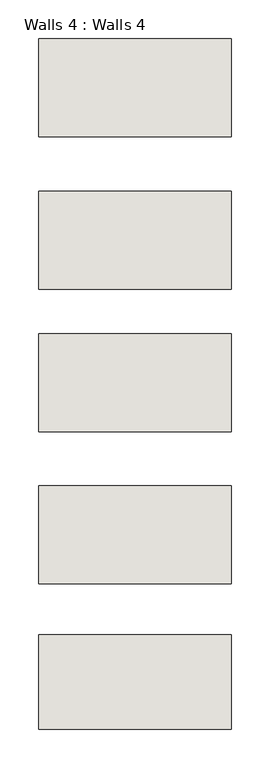
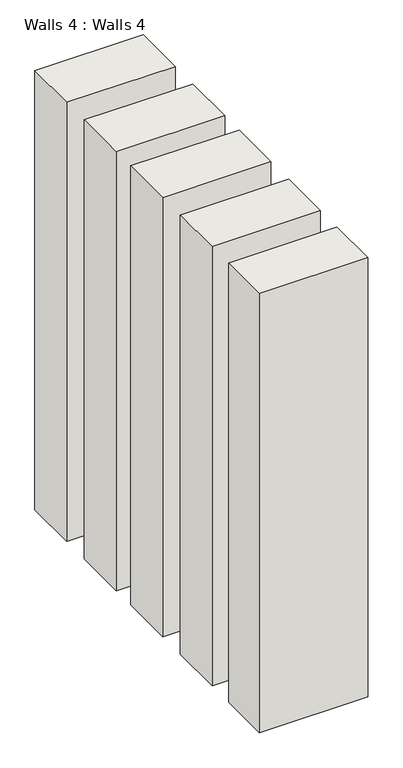
"""IFC4 building model written with IfcOpenShell, lengths in millimetres: wall geometry, Walls 4 : Walls 4."""

from ifc_helpers import new_model, si_unit, frame, origin, place, context, project, spatial, polyline, outline, extrude, source, transform, mapped, element, save


def walls_4_walls_4_d362682a(model_context):
    return source(origin(), model_context, "Body", "SweptSolid", [
        extrude(outline(polyline([(-12417.7987464, 8615.2733121), (-12417.7987464, 8488.5096557), (-12666.6001756, 8488.5096557), (-12666.6001756, 8615.2733121), (-12417.7987464, 8615.2733121)])), frame((0.0, 0.0, 9337.9259315), z_axis=(0.0, 0.0, 1.0), x_axis=(1.0, 0.0, 0.0)), (0.0, 0.0, 1.0), 1066.8),
        extrude(outline(polyline([(-12417.7987464, 8418.3217458), (-12417.7987464, 8291.5580895), (-12666.6001756, 8291.5580895), (-12666.6001756, 8418.3217458), (-12417.7987464, 8418.3217458)])), frame((0.0, 0.0, 9337.9259315), z_axis=(0.0, 0.0, 1.0), x_axis=(1.0, 0.0, 0.0)), (0.0, 0.0, 1.0), 1066.8),
        extrude(outline(polyline([(-12417.7987464, 8225.7423334), (-12417.7987464, 8103.9569405), (-12666.6001756, 8103.9569405), (-12666.6001756, 8225.7423334), (-12417.7987464, 8225.7423334)])), frame((0.0, 0.0, 9337.9259315), z_axis=(0.0, 0.0, 1.0), x_axis=(1.0, 0.0, 0.0)), (0.0, 0.0, 1.0), 1066.8),
        extrude(outline(polyline([(-12417.7987464, 8996.2733121), (-12417.7987464, 8869.5096557), (-12666.6001756, 8869.5096557), (-12666.6001756, 8996.2733121), (-12417.7987464, 8996.2733121)])), frame((0.0, 0.0, 9337.9259315), z_axis=(0.0, 0.0, 1.0), x_axis=(1.0, 0.0, 0.0)), (0.0, 0.0, 1.0), 1066.8),
        extrude(outline(polyline([(-12417.7987464, 8799.3217458), (-12417.7987464, 8672.5580895), (-12666.6001756, 8672.5580895), (-12666.6001756, 8799.3217458), (-12417.7987464, 8799.3217458)])), frame((0.0, 0.0, 9337.9259315), z_axis=(0.0, 0.0, 1.0), x_axis=(1.0, 0.0, 0.0)), (0.0, 0.0, 1.0), 1066.8),
    ])


if __name__ == "__main__":
    model = new_model("IFC4")
    model_context = context("Model", 3, world=origin())
    ifc_project = project(units=[si_unit("LENGTHUNIT", "METRE", prefix="MILLI")], contexts=[model_context])
    site = spatial("IfcSite", under=ifc_project)
    building = spatial("IfcBuilding", under=site)
    placement = place(None, origin())
    walls_4_walls_4_shape = walls_4_walls_4_d362682a(model_context)
    element("IfcWall", 1, ObjectType="Walls 4 : Walls 4", at=placement, inside=building, context=model_context, shape_type="MappedRepresentation", body=[
        mapped(walls_4_walls_4_shape, transform((0.0, 0.0, 0.0), x_axis=(1.0, 0.0, 0.0), y_axis=(0.0, 1.0, 0.0), z_axis=(0.0, 0.0, 1.0))),
    ])
    save(model, "model.ifc")

# Revit data of these elements
# Element 1 (IfcWall, "Walls 4 : Walls 4")
#   Materials on its faces: "Default Wall"
# Materials
#   "Default Wall": colour RGB 128 128 128, transparency 0
